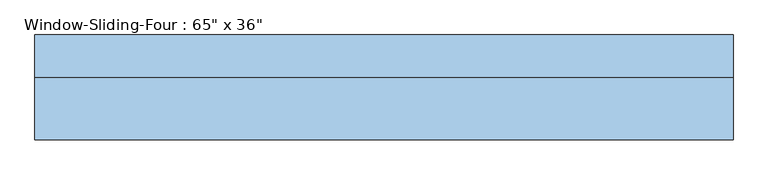
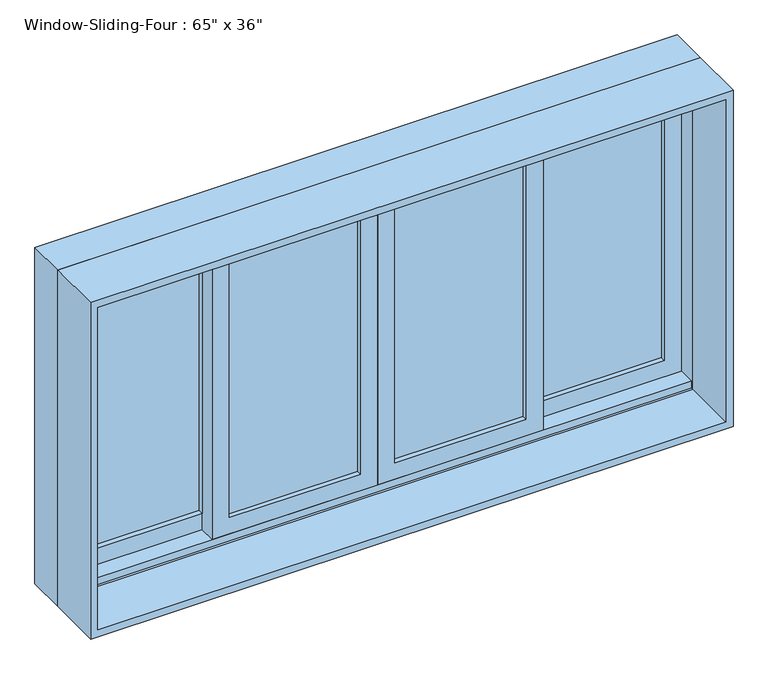
"""IFC4 building model written with IfcOpenShell, lengths in millimetres: window geometry."""

from ifc_helpers import new_model, si_unit, frame, origin, place, context, project, spatial, polyline, outline, extrude, faceted_brep, source, transform, mapped, element, save


def window_95c4569f(model_context):
    return source(origin(), model_context, "Body", "SolidModel", [
        extrude(outline(polyline([(933.45, -806.45), (933.45, -381.0), (1809.75, -381.0), (1809.75, -806.45), (933.45, -806.45)]), holes=[polyline([(1765.3, -425.45), (996.95, -425.45), (996.95, -762.0), (1765.3, -762.0), (1765.3, -425.45)])]), frame((0.0, 78.74, 0.0), z_axis=(0.0, 1.0, 0.0), x_axis=(0.0, 0.0, 1.0)), (0.0, 0.0, 1.0), 44.45),
        extrude(outline(polyline([(-425.45, 110.49), (-425.45, 104.14), (-762.0, 104.14), (-762.0, 110.49), (-425.45, 110.49)])), frame((0.0, 0.0, 996.95), z_axis=(0.0, 0.0, 1.0), x_axis=(1.0, 0.0, 0.0)), (0.0, 0.0, 1.0), 768.35),
        extrude(outline(polyline([(-425.45, 97.79), (-425.45, 91.44), (-762.0, 91.44), (-762.0, 97.79), (-425.45, 97.79)])), frame((0.0, 0.0, 996.95), z_axis=(0.0, 0.0, 1.0), x_axis=(1.0, 0.0, 0.0)), (0.0, 0.0, 1.0), 768.35),
        extrude(outline(polyline([(-44.45, 66.04), (-44.45, 59.69), (-381.0, 59.69), (-381.0, 66.04), (-44.45, 66.04)])), frame((0.0, 0.0, 996.95), z_axis=(0.0, 0.0, 1.0), x_axis=(1.0, 0.0, 0.0)), (0.0, 0.0, 1.0), 768.35),
        extrude(outline(polyline([(-44.45, 53.34), (-44.45, 46.99), (-381.0, 46.99), (-381.0, 53.34), (-44.45, 53.34)])), frame((0.0, 0.0, 996.95), z_axis=(0.0, 0.0, 1.0), x_axis=(1.0, 0.0, 0.0)), (0.0, 0.0, 1.0), 768.35),
        extrude(outline(polyline([(1828.8, -825.5), (914.4, -825.5), (914.4, 825.5), (1828.8, 825.5), (1828.8, -825.5)]), holes=[polyline([(1809.75, 806.45), (933.45, 806.45), (933.45, -806.45), (1809.75, -806.45), (1809.75, 806.45)])]), frame((0.0, -118.11, 0.0), z_axis=(0.0, 1.0, 0.0), x_axis=(0.0, 0.0, 1.0)), (0.0, 0.0, 1.0), 146.05),
        extrude(outline(polyline([(952.5, 425.45), (1809.75, 425.45), (1809.75, 0.0), (952.5, 0.0), (952.5, 425.45)]), holes=[polyline([(996.95, 44.45), (1765.3, 44.45), (1765.3, 381.0), (996.95, 381.0), (996.95, 44.45)])]), frame((0.0, 34.29, 0.0), z_axis=(0.0, 1.0, 0.0), x_axis=(0.0, 0.0, 1.0)), (0.0, 0.0, 1.0), 44.45),
        extrude(outline(polyline([(1809.75, -425.45), (952.5, -425.45), (952.5, 0.0), (1809.75, 0.0), (1809.75, -425.45)]), holes=[polyline([(1765.3, -44.45), (996.95, -44.45), (996.95, -381.0), (1765.3, -381.0), (1765.3, -44.45)])]), frame((0.0, 34.29, 0.0), z_axis=(0.0, 1.0, 0.0), x_axis=(0.0, 0.0, 1.0)), (0.0, 0.0, 1.0), 44.45),
        extrude(outline(polyline([(381.0, 66.04), (381.0, 59.69), (44.45, 59.69), (44.45, 66.04), (381.0, 66.04)])), frame((0.0, 0.0, 996.95), z_axis=(0.0, 0.0, 1.0), x_axis=(1.0, 0.0, 0.0)), (0.0, 0.0, 1.0), 768.35),
        extrude(outline(polyline([(381.0, 53.34), (381.0, 46.99), (44.45, 46.99), (44.45, 53.34), (381.0, 53.34)])), frame((0.0, 0.0, 996.95), z_axis=(0.0, 0.0, 1.0), x_axis=(1.0, 0.0, 0.0)), (0.0, 0.0, 1.0), 768.35),
        extrude(outline(polyline([(762.0, 110.49), (762.0, 104.14), (425.45, 104.14), (425.45, 110.49), (762.0, 110.49)])), frame((0.0, 0.0, 996.95), z_axis=(0.0, 0.0, 1.0), x_axis=(1.0, 0.0, 0.0)), (0.0, 0.0, 1.0), 768.35),
        extrude(outline(polyline([(762.0, 97.4725303), (762.0, 91.44), (425.45, 91.44), (425.45, 97.4725303), (762.0, 97.4725303)])), frame((0.0, 0.0, 996.95), z_axis=(0.0, 0.0, 1.0), x_axis=(1.0, 0.0, 0.0)), (0.0, 0.0, 1.0), 768.35),
        extrude(outline(polyline([(933.45, 806.45), (1809.75, 806.45), (1809.75, 381.0), (933.45, 381.0), (933.45, 806.45)]), holes=[polyline([(1765.3, 425.45), (1765.3, 762.0), (996.95, 762.0), (996.95, 425.45), (1765.3, 425.45)])]), frame((0.0, 78.74, 0.0), z_axis=(0.0, 1.0, 0.0), x_axis=(0.0, 0.0, 1.0)), (0.0, 0.0, 1.0), 44.45),
        faceted_brep([(-825.5, 27.94, 914.4), (-825.5, 129.54, 914.4), (825.5, 129.54, 914.4), (825.5, 27.94, 914.4), (-784.5778905, 129.54, 1787.8778905), (-784.5778905, 123.19, 1787.8778905), (-784.5778905, 123.19, 933.45), (-784.5778905, 129.54, 933.45), (784.5778905, 123.19, 1787.8778905), (784.5778905, 123.19, 933.45), (806.45, 123.19, 933.45), (806.45, 123.19, 1809.75), (-806.45, 123.19, 1809.75), (-806.45, 123.19, 933.45), (-806.45, 27.94, 1809.75), (-806.45, 27.94, 933.45), (-806.45, 34.29, 933.45), (-806.45, 34.29, 952.5), (-806.45, 78.74, 952.5), (-806.45, 78.74, 933.45), (825.5, 27.94, 1828.8), (-825.5, 27.94, 1828.8), (806.45, 27.94, 1809.75), (806.45, 27.94, 933.45), (-825.5, 129.54, 1828.8), (825.5, 129.54, 1828.8), (784.5778905, 129.54, 933.45), (784.5778905, 129.54, 1787.8778905), (806.45, 78.74, 933.45), (806.45, 78.74, 952.5), (806.45, 34.29, 952.5), (806.45, 34.29, 933.45)], [[[0, 1, 2, 3]], [[4, 5, 6, 7]], [[5, 8, 9, 10, 11, 12, 13, 6]], [[12, 14, 15, 16, 17, 18, 19, 13]], [[0, 3, 20, 21], [22, 23, 15, 14]], [[24, 1, 0, 21]], [[2, 1, 24, 25], [4, 7, 26, 27]], [[5, 4, 27, 8]], [[12, 11, 22, 14]], [[21, 20, 25, 24]], [[8, 27, 26, 9]], [[22, 11, 10, 28, 29, 30, 31, 23]], [[20, 3, 2, 25]], [[26, 7, 6, 13, 19, 28, 10, 9]], [[28, 19, 18, 29]], [[29, 18, 17, 30]], [[30, 17, 16, 31]], [[15, 23, 31, 16]]]),
    ])


if __name__ == "__main__":
    model = new_model("IFC4")
    model_context = context("Model", 3, world=origin())
    ifc_project = project(units=[si_unit("LENGTHUNIT", "METRE", prefix="MILLI")], contexts=[model_context])
    site = spatial("IfcSite", under=ifc_project)
    building = spatial("IfcBuilding", under=site)
    placement = place(None, origin())
    window_shape = window_95c4569f(model_context)
    element("IfcWindow", 1, ObjectType="Window-Sliding-Four : 65\" x 36\"", at=placement, inside=building, context=model_context, shape_type="MappedRepresentation", body=[
        mapped(window_shape, transform((0.0, 0.0, 0.0), x_axis=(1.0, 0.0, 0.0), y_axis=(0.0, 1.0, 0.0), z_axis=(0.0, 0.0, 1.0))),
    ])
    save(model, "model.ifc")

# Revit data of these elements
# Type "Window-Sliding-Four : 65\" x 36\""
#   Type Mark = "19"
#   Fire Rating = "0.5h"
#   Assembly Code = "B2020100"
#   Analytic Construction = "Double glazing - domestic"
#   Window Inset [instance default] = 0' - 0"
#   Wall Thickness [instance default] = 0' - 6"
#   Visual Light Transmittance = 0.81
#   Thermal Resistance (R) = 1.8146 (h·ft²·°F)/BTU
#   Solar Heat Gain Coefficient = 0.76
#   Interior Wall Closure [instance default] = 0' - 2 19/32"
#   Heat Transfer Coefficient (U) = 0.5511 BTU/(h·ft²·°F)
#   Frame Extension [instance default] = 0' - 0 1/4"
#   Exterior Wall Closure [instance default] = 0' - 1 1/4"
#   Rough Width = 5' - 5 1/2"
#   Rough Height = 3' - 0 1/2"
#   Height = 3' - 0"
#   Extension Jamb [instance default] = 0' - 2 3/4"
#   Default Sill Height = 3' - 0"
#   Width = 5' - 5"
#   Middle Muntin Visibility = yes
#   Interior Trim Visibility [instance default] = yes
#   Indicator Visibility [instance default] = yes
#   Exterior Trim Visibility [instance default] = yes
#   Side Muntin Visibility = yes
#   Extension Jamb Visibility [instance default] = yes
#   Interior Trim Material = Wood - Stained
#   Muntin Pattern = Muntin Pattern_2x2 : Muntin Pattern_2x2
#   Interior Trim = Trim-Window-Interior-Flat : Picture Frame
#   Interior Frame Material = Wood - Stained
#   Glass Panel Material = Glass
#   Exterior Trim Material = Clad - White
#   Exterior Trim = Trim-Window-Exterior-Flat : with Sill
#   Exterior Frame Material = Clad - White
#   Wall Closure = (empty or 0)
# Element 1 (IfcWindow, "Window-Sliding-Four : 65\" x 36\"")
#   Wall Thickness = 0' - 9"
#   Interior Wall Closure = 0' - 2 3/4"
#   Extension Jamb = 0' - 5 3/4"
#   Materials on its faces: "Wood - Stained", "Glass", "Clad - White"
# Materials
#   "Wood - Stained": class "Wood", colour RGB 224 178 126, transparency 0, Cost = 0
#   "Glass": class "Glass", colour RGB 0 128 192, transparency 0.75, Description = "Soda Lime Glass", Cost = 0
#   "Clad - White": class "Wood", colour RGB 242 242 238, transparency 0, Cost = 0
